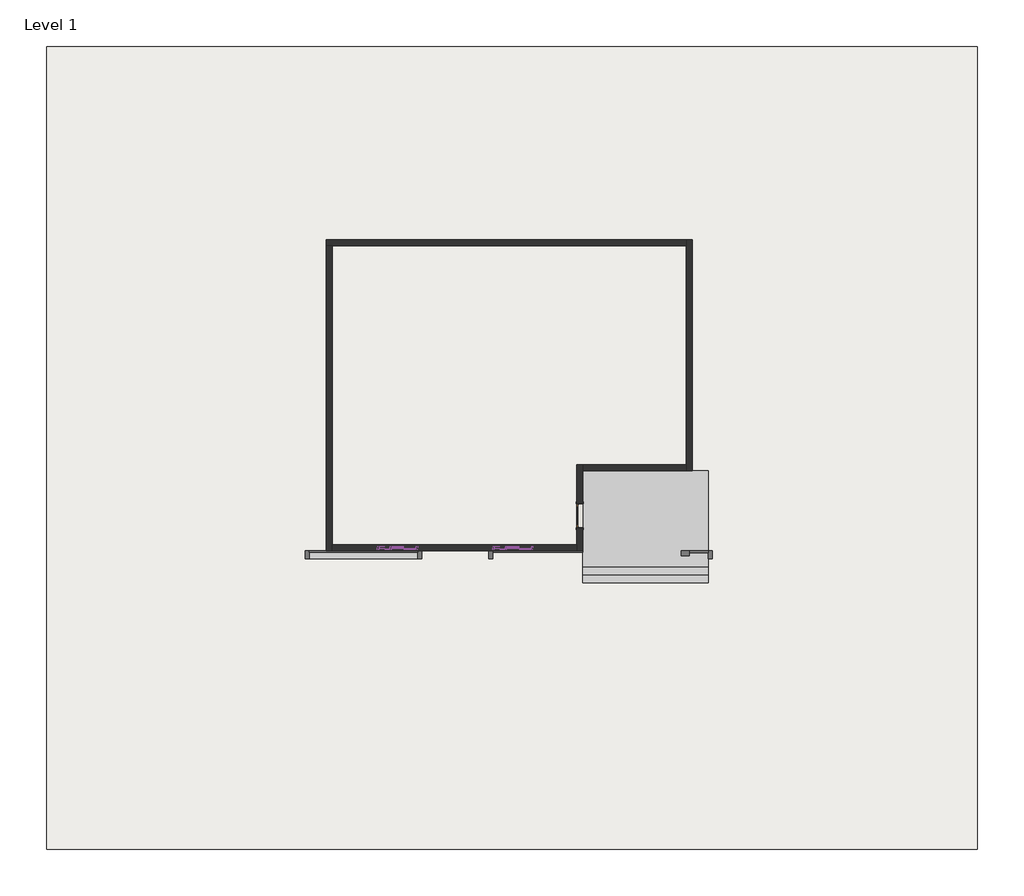
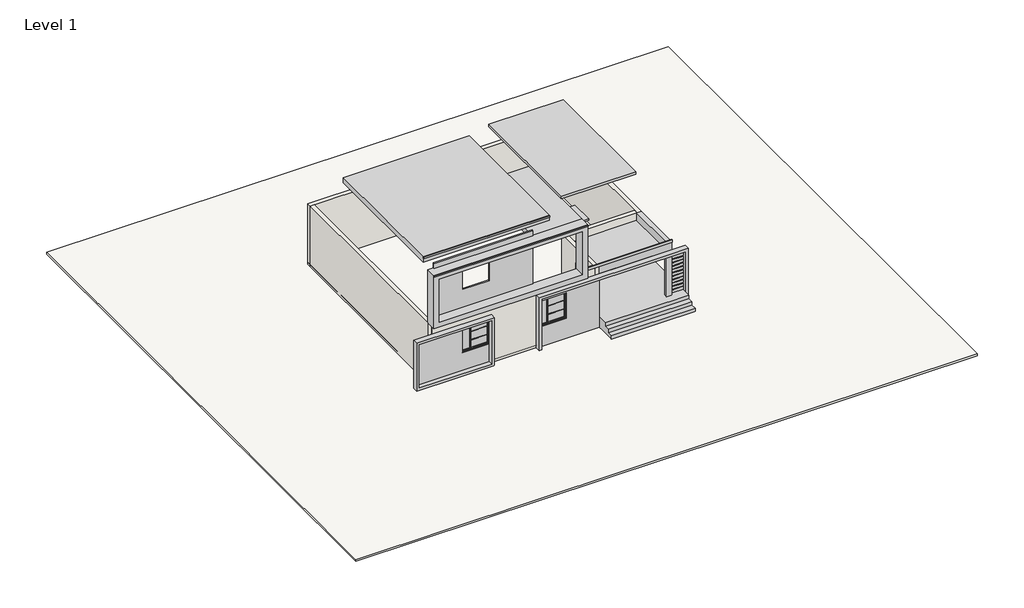
# One storey: 30 members, 8 plates, 6 walls, 2 slabs, 1 door, 1 proxy.
"""IFC4 building model written with IfcOpenShell, lengths in millimetres."""

from ifc_helpers import new_model, si_unit, frame, origin, origin_with_axes, place, context, project, spatial, polyline, outline, extrude, faceted_brep, transform, mapped, element, save
from components import generic_models_1_generic_models_1_b41e56dc, door_interior_single_1_panel_wood_4_x7_868ee8a9, member_c9b54d35, member_90750a43, member_dc106669, member_ff82125d, member_7fd687a9, system_panel_glazed_5efa86ec, system_panel_glazed_26b8bff8, system_panel_glazed_31531e99

model = new_model("IFC4")

# Units and contexts
model_context = context("Model", 3, world=origin())
ifc_project = project(units=[si_unit("LENGTHUNIT", "METRE", prefix="MILLI")], contexts=[model_context])

# Site, building, storey
site = spatial("IfcSite", under=ifc_project)
building = spatial("IfcBuilding", under=site)
storey = spatial("IfcBuildingStorey", under=building, Name="Level 1", Elevation=0.0)

# Proxy
placement = place(None, origin())
generic_models_1_generic_models_1_shape = generic_models_1_generic_models_1_b41e56dc(model_context)
element("IfcBuildingElementProxy", 1, Name="Generic Models 1 : Generic Models 1", ObjectType="Generic Models 1 : Generic Models 1", at=placement, inside=storey, context=model_context, shape_type="MappedRepresentation", body=[
    mapped(generic_models_1_generic_models_1_shape, transform((0.0, 0.0, 0.0), x_axis=(1.0, 0.0, 0.0), y_axis=(0.0, 1.0, 0.0), z_axis=(0.0, 0.0, 1.0))),
])

# Door
door_interior_single_1_panel_wood_4_x7_shape = door_interior_single_1_panel_wood_4_x7_868ee8a9(model_context)
element("IfcDoor", 2, ObjectType="Door-Interior-Single-1_Panel-Wood : 4'x7'", at=placement, inside=storey, context=model_context, shape_type="MappedRepresentation", body=[
    mapped(door_interior_single_1_panel_wood_4_x7_shape, transform((1261.9006121, -1809.8883122, 609.6), x_axis=(0.0, -1.0, 0.0), y_axis=(1.0, 0.0, 0.0), z_axis=(0.0, 0.0, 1.0))),
])

# Members
member_shape = member_c9b54d35(model_context)
element("IfcMember", 3, ObjectType="Rectangular Mullion : 1.5\" x 2.5\" rectangular", at=placement, inside=storey, context=model_context, shape_type="MappedRepresentation", body=[
    mapped(member_shape, transform((-5878.6743879, -3029.0883122, 2235.2), x_axis=(0.0, 0.0, 1.0), y_axis=(0.0, 1.0, 0.0), z_axis=(-1.0, 0.0, 0.0))),
])
element("IfcMember", 4, ObjectType="Rectangular Mullion : 1.5\" x 2.5\" rectangular", at=placement, inside=storey, context=model_context, shape_type="MappedRepresentation", body=[
    mapped(member_shape, transform((-5878.6743879, -3029.0883122, 1727.2), x_axis=(0.0, 0.0, 1.0), y_axis=(0.0, 1.0, 0.0), z_axis=(-1.0, 0.0, 0.0))),
])
element("IfcMember", 5, ObjectType="Rectangular Mullion : 1.5\" x 2.5\" rectangular", at=placement, inside=storey, context=model_context, shape_type="MappedRepresentation", body=[
    mapped(member_shape, transform((-1497.1743879, -3029.0883122, 2235.2), x_axis=(0.0, 0.0, 1.0), y_axis=(0.0, 1.0, 0.0), z_axis=(-1.0, 0.0, 0.0))),
])
element("IfcMember", 6, ObjectType="Rectangular Mullion : 1.5\" x 2.5\" rectangular", at=placement, inside=storey, context=model_context, shape_type="MappedRepresentation", body=[
    mapped(member_shape, transform((-1497.1743879, -3029.0883122, 1727.2), x_axis=(0.0, 0.0, 1.0), y_axis=(0.0, 1.0, 0.0), z_axis=(-1.0, 0.0, 0.0))),
])
member_2_shape = member_90750a43(model_context)
element("IfcMember", 7, ObjectType="Rectangular Mullion : 2.5\" x 5\" rectangular", at=placement, inside=storey, context=model_context, shape_type="MappedRepresentation", body=[
    mapped(member_2_shape, transform((-5910.4243879, -3029.0883122, 1727.2), x_axis=(-1.0, 0.0, 0.0), y_axis=(0.0, 1.0, 0.0), z_axis=(0.0, 0.0, -1.0))),
])
element("IfcMember", 8, ObjectType="Rectangular Mullion : 2.5\" x 5\" rectangular", at=placement, inside=storey, context=model_context, shape_type="MappedRepresentation", body=[
    mapped(member_2_shape, transform((-1528.9243879, -3029.0883122, 1727.2), x_axis=(-1.0, 0.0, 0.0), y_axis=(0.0, 1.0, 0.0), z_axis=(0.0, 0.0, -1.0))),
])
element("IfcMember", 9, ObjectType="Rectangular Mullion : 2.5\" x 5\" rectangular", at=placement, inside=storey, context=model_context, shape_type="MappedRepresentation", body=[
    mapped(member_2_shape, transform((-5910.4243879, -3029.0883122, 2235.2), x_axis=(-1.0, 0.0, 0.0), y_axis=(0.0, 1.0, 0.0), z_axis=(0.0, 0.0, -1.0))),
])
element("IfcMember", 10, ObjectType="Rectangular Mullion : 2.5\" x 5\" rectangular", at=placement, inside=storey, context=model_context, shape_type="MappedRepresentation", body=[
    mapped(member_2_shape, transform((-1528.9243879, -3029.0883122, 2235.2), x_axis=(-1.0, 0.0, 0.0), y_axis=(0.0, 1.0, 0.0), z_axis=(0.0, 0.0, -1.0))),
])
element("IfcMember", 11, ObjectType="Rectangular Mullion : 2.5\" x 5\" rectangular", at=placement, inside=storey, context=model_context, shape_type="MappedRepresentation", body=[
    mapped(member_2_shape, transform((-5910.4243879, -3029.0883122, 1219.2), x_axis=(-1.0, 0.0, 0.0), y_axis=(0.0, 1.0, 0.0), z_axis=(0.0, 0.0, -1.0))),
])
element("IfcMember", 12, ObjectType="Rectangular Mullion : 2.5\" x 5\" rectangular", at=placement, inside=storey, context=model_context, shape_type="MappedRepresentation", body=[
    mapped(member_2_shape, transform((-1528.9243879, -3029.0883122, 1219.2), x_axis=(-1.0, 0.0, 0.0), y_axis=(0.0, 1.0, 0.0), z_axis=(0.0, 0.0, -1.0))),
])
member_3_shape = member_dc106669(model_context)
element("IfcMember", 13, ObjectType="Rectangular Mullion : 2.5\" x 5\" rectangular", at=placement, inside=storey, context=model_context, shape_type="MappedRepresentation", body=[
    mapped(member_3_shape, transform((-6354.9243879, -3029.0883122, 2743.2), x_axis=(0.0, 0.0, 1.0), y_axis=(0.0, 1.0, 0.0), z_axis=(-1.0, 0.0, 0.0))),
])
element("IfcMember", 14, ObjectType="Rectangular Mullion : 2.5\" x 5\" rectangular", at=placement, inside=storey, context=model_context, shape_type="MappedRepresentation", body=[
    mapped(member_3_shape, transform((-1973.4243879, -3029.0883122, 2743.2), x_axis=(0.0, 0.0, 1.0), y_axis=(0.0, 1.0, 0.0), z_axis=(-1.0, 0.0, 0.0))),
])
member_4_shape = member_ff82125d(model_context)
element("IfcMember", 15, ObjectType="Rectangular Mullion : 2.5\" x 5\" rectangular", at=placement, inside=storey, context=model_context, shape_type="MappedRepresentation", body=[
    mapped(member_4_shape, transform((-4957.9243879, -3029.0883122, 1219.2), x_axis=(0.0, 0.0, -1.0), y_axis=(0.0, 1.0, 0.0), z_axis=(1.0, 0.0, 0.0))),
])
element("IfcMember", 16, ObjectType="Rectangular Mullion : 2.5\" x 5\" rectangular", at=placement, inside=storey, context=model_context, shape_type="MappedRepresentation", body=[
    mapped(member_4_shape, transform((-576.4243879, -3029.0883122, 1219.2), x_axis=(0.0, 0.0, -1.0), y_axis=(0.0, 1.0, 0.0), z_axis=(1.0, 0.0, 0.0))),
])
element("IfcMember", 17, ObjectType="Rectangular Mullion : 2.5\" x 5\" rectangular", at=placement, inside=storey, context=model_context, shape_type="MappedRepresentation", body=[
    mapped(member_3_shape, transform((-5942.1743879, -3029.0883122, 1219.2), x_axis=(0.0, 0.0, -1.0), y_axis=(0.0, 1.0, 0.0), z_axis=(1.0, 0.0, 0.0))),
])
element("IfcMember", 18, ObjectType="Rectangular Mullion : 2.5\" x 5\" rectangular", at=placement, inside=storey, context=model_context, shape_type="MappedRepresentation", body=[
    mapped(member_3_shape, transform((-1560.6743879, -3029.0883122, 1219.2), x_axis=(0.0, 0.0, -1.0), y_axis=(0.0, 1.0, 0.0), z_axis=(1.0, 0.0, 0.0))),
])
element("IfcMember", 19, ObjectType="Rectangular Mullion : 2.5\" x 5\" rectangular", at=placement, inside=storey, context=model_context, shape_type="MappedRepresentation", body=[
    mapped(member_4_shape, transform((-5878.6743879, -3029.0883122, 2743.2), x_axis=(0.0, 0.0, 1.0), y_axis=(0.0, 1.0, 0.0), z_axis=(-1.0, 0.0, 0.0))),
])
element("IfcMember", 20, ObjectType="Rectangular Mullion : 2.5\" x 5\" rectangular", at=placement, inside=storey, context=model_context, shape_type="MappedRepresentation", body=[
    mapped(member_4_shape, transform((-1497.1743879, -3029.0883122, 2743.2), x_axis=(0.0, 0.0, 1.0), y_axis=(0.0, 1.0, 0.0), z_axis=(-1.0, 0.0, 0.0))),
])
member_5_shape = member_7fd687a9(model_context)
element("IfcMember", 21, ObjectType="Rectangular Mullion : 2.5\" x 5\" rectangular", at=placement, inside=storey, context=model_context, shape_type="MappedRepresentation", body=[
    mapped(member_5_shape, transform((-4894.4243879, -3029.0883122, 2743.2), x_axis=(1.0, 0.0, 0.0), y_axis=(0.0, 1.0, 0.0), z_axis=(0.0, 0.0, 1.0))),
])
element("IfcMember", 22, ObjectType="Rectangular Mullion : 2.5\" x 5\" rectangular", at=placement, inside=storey, context=model_context, shape_type="MappedRepresentation", body=[
    mapped(member_5_shape, transform((-512.9243879, -3029.0883122, 2743.2), x_axis=(1.0, 0.0, 0.0), y_axis=(0.0, 1.0, 0.0), z_axis=(0.0, 0.0, 1.0))),
])
element("IfcMember", 23, ObjectType="Rectangular Mullion : 2.5\" x 5\" rectangular", at=placement, inside=storey, context=model_context, shape_type="MappedRepresentation", body=[
    mapped(member_5_shape, transform((-6418.4243879, -3029.0883122, 1219.2), x_axis=(-1.0, 0.0, 0.0), y_axis=(0.0, 1.0, 0.0), z_axis=(0.0, 0.0, -1.0))),
])
element("IfcMember", 24, ObjectType="Rectangular Mullion : 2.5\" x 5\" rectangular", at=placement, inside=storey, context=model_context, shape_type="MappedRepresentation", body=[
    mapped(member_5_shape, transform((-2036.9243879, -3029.0883122, 1219.2), x_axis=(-1.0, 0.0, 0.0), y_axis=(0.0, 1.0, 0.0), z_axis=(0.0, 0.0, -1.0))),
])
element("IfcMember", 25, ObjectType="Rectangular Mullion : 2.5\" x 5\" rectangular", at=placement, inside=storey, context=model_context, shape_type="MappedRepresentation", body=[
    mapped(member_5_shape, transform((-6418.4243879, -3029.0883122, 2235.2), x_axis=(-1.0, 0.0, 0.0), y_axis=(0.0, 1.0, 0.0), z_axis=(0.0, 0.0, -1.0))),
])
element("IfcMember", 26, ObjectType="Rectangular Mullion : 2.5\" x 5\" rectangular", at=placement, inside=storey, context=model_context, shape_type="MappedRepresentation", body=[
    mapped(member_5_shape, transform((-2036.9243879, -3029.0883122, 2235.2), x_axis=(-1.0, 0.0, 0.0), y_axis=(0.0, 1.0, 0.0), z_axis=(0.0, 0.0, -1.0))),
])
element("IfcMember", 27, ObjectType="Rectangular Mullion : 2.5\" x 5\" rectangular", at=placement, inside=storey, context=model_context, shape_type="MappedRepresentation", body=[
    mapped(member_5_shape, transform((-6418.4243879, -3029.0883122, 1727.2), x_axis=(-1.0, 0.0, 0.0), y_axis=(0.0, 1.0, 0.0), z_axis=(0.0, 0.0, -1.0))),
])
element("IfcMember", 28, ObjectType="Rectangular Mullion : 2.5\" x 5\" rectangular", at=placement, inside=storey, context=model_context, shape_type="MappedRepresentation", body=[
    mapped(member_5_shape, transform((-2036.9243879, -3029.0883122, 1727.2), x_axis=(-1.0, 0.0, 0.0), y_axis=(0.0, 1.0, 0.0), z_axis=(0.0, 0.0, -1.0))),
])
element("IfcMember", 29, ObjectType="Rectangular Mullion : 2.5\" x 5\" rectangular", at=placement, inside=storey, context=model_context, shape_type="MappedRepresentation", body=[
    mapped(member_5_shape, transform((-4894.4243879, -3029.0883122, 2235.2), x_axis=(1.0, 0.0, 0.0), y_axis=(0.0, 1.0, 0.0), z_axis=(0.0, 0.0, 1.0))),
])
element("IfcMember", 30, ObjectType="Rectangular Mullion : 2.5\" x 5\" rectangular", at=placement, inside=storey, context=model_context, shape_type="MappedRepresentation", body=[
    mapped(member_5_shape, transform((-512.9243879, -3029.0883122, 2235.2), x_axis=(1.0, 0.0, 0.0), y_axis=(0.0, 1.0, 0.0), z_axis=(0.0, 0.0, 1.0))),
])
element("IfcMember", 31, ObjectType="Rectangular Mullion : 2.5\" x 5\" rectangular", at=placement, inside=storey, context=model_context, shape_type="MappedRepresentation", body=[
    mapped(member_5_shape, transform((-4894.4243879, -3029.0883122, 1727.2), x_axis=(1.0, 0.0, 0.0), y_axis=(0.0, 1.0, 0.0), z_axis=(0.0, 0.0, 1.0))),
])
element("IfcMember", 32, ObjectType="Rectangular Mullion : 2.5\" x 5\" rectangular", at=placement, inside=storey, context=model_context, shape_type="MappedRepresentation", body=[
    mapped(member_5_shape, transform((-512.9243879, -3029.0883122, 1727.2), x_axis=(1.0, 0.0, 0.0), y_axis=(0.0, 1.0, 0.0), z_axis=(0.0, 0.0, 1.0))),
])

# Plates
system_panel_glazed_shape = system_panel_glazed_5efa86ec(model_context)
element("IfcPlate", 33, ObjectType="System Panel : Glazed", at=placement, inside=storey, context=model_context, shape_type="MappedRepresentation", body=[
    mapped(system_panel_glazed_shape, transform((-1036.7993879, -3029.0883122, 1282.7), x_axis=(-1.0, 0.0, 0.0), y_axis=(0.0, -1.0, 0.0), z_axis=(0.0, 0.0, 1.0))),
])
element("IfcPlate", 34, ObjectType="System Panel : Glazed", at=placement, inside=storey, context=model_context, shape_type="MappedRepresentation", body=[
    mapped(system_panel_glazed_shape, transform((-5418.2993879, -3029.0883122, 1282.7), x_axis=(-1.0, 0.0, 0.0), y_axis=(0.0, -1.0, 0.0), z_axis=(0.0, 0.0, 1.0))),
])
element("IfcPlate", 35, ObjectType="System Panel : Glazed", at=placement, inside=storey, context=model_context, shape_type="MappedRepresentation", body=[
    mapped(system_panel_glazed_shape, transform((-5418.2993879, -3029.0883122, 2254.25), x_axis=(-1.0, 0.0, 0.0), y_axis=(0.0, -1.0, 0.0), z_axis=(0.0, 0.0, 1.0))),
])
element("IfcPlate", 36, ObjectType="System Panel : Glazed", at=placement, inside=storey, context=model_context, shape_type="MappedRepresentation", body=[
    mapped(system_panel_glazed_shape, transform((-1036.7993879, -3029.0883122, 2254.25), x_axis=(-1.0, 0.0, 0.0), y_axis=(0.0, -1.0, 0.0), z_axis=(0.0, 0.0, 1.0))),
])
system_panel_glazed_2_shape = system_panel_glazed_26b8bff8(model_context)
element("IfcPlate", 37, ObjectType="System Panel : Glazed", at=placement, inside=storey, context=model_context, shape_type="MappedRepresentation", body=[
    mapped(system_panel_glazed_2_shape, transform((-6148.5493879, -3029.0883122, 1282.7), x_axis=(-1.0, 0.0, 0.0), y_axis=(0.0, -1.0, 0.0), z_axis=(0.0, 0.0, 1.0))),
])
element("IfcPlate", 38, ObjectType="System Panel : Glazed", at=placement, inside=storey, context=model_context, shape_type="MappedRepresentation", body=[
    mapped(system_panel_glazed_2_shape, transform((-1767.0493879, -3029.0883122, 1282.7), x_axis=(-1.0, 0.0, 0.0), y_axis=(0.0, -1.0, 0.0), z_axis=(0.0, 0.0, 1.0))),
])
system_panel_glazed_3_shape = system_panel_glazed_31531e99(model_context)
element("IfcPlate", 39, ObjectType="System Panel : Glazed", at=placement, inside=storey, context=model_context, shape_type="MappedRepresentation", body=[
    mapped(system_panel_glazed_3_shape, transform((-5418.2993879, -3029.0883122, 1746.25), x_axis=(-1.0, 0.0, 0.0), y_axis=(0.0, -1.0, 0.0), z_axis=(0.0, 0.0, 1.0))),
])
element("IfcPlate", 40, ObjectType="System Panel : Glazed", at=placement, inside=storey, context=model_context, shape_type="MappedRepresentation", body=[
    mapped(system_panel_glazed_3_shape, transform((-1036.7993879, -3029.0883122, 1746.25), x_axis=(-1.0, 0.0, 0.0), y_axis=(0.0, -1.0, 0.0), z_axis=(0.0, 0.0, 1.0))),
])

# Slabs
element("IfcSlab", 41, ObjectType="4\" floor", at=placement, inside=storey, context=model_context, shape_type="SweptSolid", body=[
    extrude(outline(polyline([(16371.8639765, 16010.8782458), (16371.8639765, -14469.1217542), (-18984.9360235, -14469.1217542), (-18984.9360235, 16010.8782458), (16371.8639765, 16010.8782458)])), frame((0.0, 0.0, -101.6), z_axis=(0.0, 0.0, 1.0), x_axis=(1.0, 0.0, 0.0)), (0.0, 0.0, 1.0), 101.6),
])
element("IfcSlab", 42, ObjectType="6\" GF", at=placement, inside=storey, context=model_context, shape_type="SweptSolid", body=[
    extrude(outline(polyline([(5532.2756121, 8667.6116878), (5532.2756121, -3143.3883122), (-8361.5243879, -3143.3883122), (-8361.5243879, 8667.6116878), (5532.2756121, 8667.6116878)])), origin_with_axes(), (0.0, 0.0, 1.0), 152.4),
])

# Walls
element("IfcWall", 43, ObjectType="9\" wall", at=placement, inside=storey, context=model_context, shape_type="Brep", body=[
    faceted_brep([(-8361.5243879, 8439.0116878, 0.0), (-8132.9243879, 8439.0116878, 0.0), (5303.6756121, 8439.0116878, 0.0), (5303.6756121, 8439.0116878, 3657.6), (-8132.9243879, 8439.0116878, 3657.6), (-8361.5243879, 8439.0116878, 3657.6), (-8361.5243879, 8667.6116878, 0.0), (-8361.5243879, 8667.6116878, 3657.6), (5303.6756121, 8667.6116878, 3657.6), (5303.6756121, 8667.6116878, 0.0)], [[[0, 1, 2, 3, 4, 5]], [[6, 7, 8, 9]], [[2, 1, 0, 6, 9]], [[5, 4, 3, 8, 7]], [[0, 5, 7, 6]], [[3, 2, 9, 8]]]),
])
element("IfcWall", 44, ObjectType="9\" wall", at=placement, inside=storey, context=model_context, shape_type="Brep", body=[
    faceted_brep([(-8132.9243879, -3143.3883122, 0.0), (-8132.9243879, -2914.7883122, 0.0), (-8132.9243879, 8439.0116878, 0.0), (-8132.9243879, 8439.0116878, 3657.6), (-8132.9243879, -2914.7883122, 3657.6), (-8132.9243879, -3143.3883122, 3657.6), (-8361.5243879, -3143.3883122, 0.0), (-8361.5243879, -3143.3883122, 3657.6), (-8361.5243879, 8439.0116878, 3657.6), (-8361.5243879, 8439.0116878, 0.0)], [[[0, 1, 2, 3, 4, 5]], [[6, 7, 8, 9]], [[2, 1, 0, 6, 9]], [[5, 4, 3, 8, 7]], [[0, 5, 7, 6]], [[3, 2, 9, 8]]]),
])
element("IfcWall", 45, ObjectType="9\" wall", at=placement, inside=storey, context=model_context, shape_type="Brep", body=[
    faceted_brep([(5303.6756121, 8667.6116878, 0.0), (5303.6756121, 8439.0116878, 0.0), (5303.6756121, 133.2116878, 0.0), (5303.6756121, -95.3883122, 0.0), (5303.6756121, -95.3883122, 3657.6), (5303.6756121, 133.2116878, 3657.6), (5303.6756121, 8439.0116878, 3657.6), (5303.6756121, 8667.6116878, 3657.6), (5532.2756121, 8667.6116878, 0.0), (5532.2756121, 8667.6116878, 3657.6), (5532.2756121, -95.3883122, 3657.6), (5532.2756121, -95.3883122, 0.0)], [[[0, 1, 2, 3, 4, 5, 6, 7]], [[8, 9, 10, 11]], [[3, 2, 1, 0, 8, 11]], [[7, 6, 5, 4, 10, 9]], [[0, 7, 9, 8]], [[4, 3, 11, 10]]]),
])
element("IfcWall", 46, ObjectType="9\" wall", at=placement, inside=storey, context=model_context, shape_type="Brep", body=[
    faceted_brep([(1379.3756121, -3143.3883122, 0.0), (1379.3756121, -95.3883122, 0.0), (1379.3756121, 133.2116878, 0.0), (1379.3756121, 133.2116878, 3657.6), (1379.3756121, -95.3883122, 3657.6), (1379.3756121, -3143.3883122, 3657.6), (1379.3756121, -2292.4883122, 609.6), (1379.3756121, -2292.4883122, 2768.6), (1379.3756121, -1327.2883122, 2768.6), (1379.3756121, -1327.2883122, 609.6), (1150.7756121, 133.2116878, 0.0), (1150.7756121, -2914.7883122, 0.0), (1150.7756121, -3143.3883122, 0.0), (1150.7756121, -3143.3883122, 3657.6), (1150.7756121, -2914.7883122, 3657.6), (1150.7756121, 133.2116878, 3657.6), (1150.7756121, -2292.4883122, 2768.6), (1150.7756121, -2292.4883122, 609.6), (1150.7756121, -1327.2883122, 609.6), (1150.7756121, -1327.2883122, 2768.6)], [[[0, 1, 2, 3, 4, 5], [6, 7, 8, 9]], [[10, 11, 12, 13, 14, 15], [16, 17, 18, 19]], [[2, 1, 0, 12, 11, 10]], [[5, 4, 3, 15, 14, 13]], [[3, 2, 10, 15]], [[0, 5, 13, 12]], [[6, 17, 16, 7]], [[7, 16, 19, 8]], [[8, 19, 18, 9]], [[17, 6, 9, 18]]]),
])
element("IfcWall", 47, ObjectType="9\" wall", at=placement, inside=storey, context=model_context, shape_type="SweptSolid", body=[
    extrude(outline(polyline([(5303.6756121, -95.3883122), (1379.3756121, -95.3883122), (1379.3756121, 133.2116878), (5303.6756121, 133.2116878), (5303.6756121, -95.3883122)])), origin_with_axes(), (0.0, 0.0, 1.0), 3657.6),
])
element("IfcWall", 48, ObjectType="9\" wall", at=placement, inside=storey, context=model_context, shape_type="SweptSolid", body=[
    extrude(outline(polyline([(0.0, -8132.9243879), (0.0, 1150.7756121), (3657.6, 1150.7756121), (3657.6, -8132.9243879), (0.0, -8132.9243879)]), holes=[polyline([(2743.2, -4894.4243879), (1219.2, -4894.4243879), (1219.2, -6418.4243879), (2743.2, -6418.4243879), (2743.2, -4894.4243879)]), polyline([(2743.2, -512.9243879), (1219.2, -512.9243879), (1219.2, -2036.9243879), (2743.2, -2036.9243879), (2743.2, -512.9243879)])]), frame((0.0, -3143.3883122, 0.0), z_axis=(0.0, 1.0, 0.0), x_axis=(0.0, 0.0, 1.0)), (0.0, 0.0, 1.0), 228.6),
])

save(model, "model.ifc")

# Revit data of these elements
# Type "Door-Interior-Single-1_Panel-Wood : 4'x7'"
#   Type Mark = "9"
#   Assembly Code = "C1020300"
#   Analytic Construction = "Wooden"
#   Top Rail = 0' - 4 11/16"
#   Thickness = 0' - 1 3/8"
#   Thermal Resistance (R) = 2.5876 (h·ft²·°F)/BTU
#   Swing Angle [instance default] = 90.00°
#   Stiles = 0' - 4 3/4"
#   Rough Width = 3' - 2"
#   Rough Height = 7' - 1"
#   Height = 7' - 0"
#   Width = 3' - 0"
#   Heat Transfer Coefficient (U) = 0.3865 BTU/(h·ft²·°F)
#   Bottom Rail = 0' - 9 1/8"
#   Trim Material = Cherry
#   Panel Material = Cherry
#   Frame Material = Cherry
#   Door Handle Material = Aluminum
#   Visual Light Transmittance = 0
#   Solar Heat Gain Coefficient = 0
#   Wall Closure = (empty or 0)
#   Function = (empty or 0)
# Type "Rectangular Mullion : 1.5\" x 2.5\" rectangular"
#   built-in parameter 1007304 = 0.208333 (stored number, unit not read)
#   built-in parameter 1007301 = 0.0625 (stored number, unit not read)
#   built-in parameter 1007300 = 0.0625 (stored number, unit not read)
# Type "Rectangular Mullion : 2.5\" x 5\" rectangular"
#   built-in parameter 1007304 = 0.416667 (stored number, unit not read)
#   built-in parameter 1007301 = 0.104167 (stored number, unit not read)
#   built-in parameter 1007300 = 0.104167 (stored number, unit not read)
# Type "System Panel : Glazed"
#   Construction Type Id = "GSP4R"
#   Analytic Construction = "1/8 in Pilkington single glazing"
#   Visual Light Transmittance = 0.9
#   Solar Heat Gain Coefficient = 0.86
#   Heat Transfer Coefficient (U) = 1.18115 BTU/(h·ft²·°F)
#   Define Thermal Properties by = 1
# Type "4\" floor"
#   Assembly Code = "B1010"
#   Function = 0
# Type "6\" GF"
#   Assembly Code = "B1010"
#   Function = 0
#   Layers, outside or top first: 0' - 6" no material (function 1)
# Type "9\" wall"
#   Assembly Code = "B2010"
#   Layers, outside or top first: 0' - 9" no material (function 1)
# Element 1 (IfcBuildingElementProxy, "Generic Models 1 : Generic Models 1")
#   Phase Created = New Construction
#   Materials on its faces: "Gypsum Wall Board", "Clad - White", "Wood Planks", "Ash colour"
# Element 2 (IfcDoor, "Door-Interior-Single-1_Panel-Wood : 4'x7'")
#   Swing Angle = 90.00°
#   Phase Created = New Construction
#   Materials on its faces: "Cherry", "Aluminum"
# Elements 3, 4, 5, 6 (IfcMember, "Rectangular Mullion : 1.5\" x 2.5\" rectangular")
#   Phase Created = New Construction
# Elements 7, 8, 9, 10, 11, 12, 13, 14, 15, 16, 17, 18, 19, 20, 21, 22, 23, 24, 25, 26, 27, 28, 29, 30, 31, 32 (IfcMember, "Rectangular Mullion : 2.5\" x 5\" rectangular")
#   Phase Created = New Construction
# Elements 33, 34, 35, 36, 37, 38, 39, 40 (IfcPlate, "System Panel : Glazed")
#   Phase Created = New Construction
#   Materials on its faces: "Glass"
# Element 41 (IfcSlab, "4\" floor")
#   Height Offset From Level = 0' - 0"
#   Phase Created = New Construction
# Element 42 (IfcSlab, "6\" GF")
#   Height Offset From Level = 0' - 6"
#   Phase Created = New Construction
#   Materials on its faces: "Default Floor"
# Elements 43, 44, 45, 46, 47, 48 (IfcWall, "9\" wall")
#   Top Offset = 0' - 0"
#   Base Offset = 0' - 0"
#   wall height = 12' - 0"
#   Phase Created = New Construction
#   Base Constraint = Level 1
#   Top Constraint = Level 2
#   Materials on its faces: "Default Wall"
# Materials
#   "Cherry": class "Wood", colour RGB 226 177 128, transparency 0, Description = "Prunus Serotina", Cost = 0
#   "Aluminum": class "Metal", colour RGB 247 247 247, transparency 0, Description = "Aluminum 6061", Cost = 0
#   "Gypsum Wall Board": class "Generic", colour RGB 127 127 127, transparency 0, Description = "Gypsum Wall Board", Cost = 0
#   "Clad - White": class "Wood", colour RGB 242 242 238, transparency 0, Cost = 0
#   "Wood Planks": class "Wood", colour RGB 193 160 115, transparency 0, Description = "Physical material.", Cost = 0
#   "Ash colour": class "Generic", colour RGB 120 120 120, transparency 0, Cost = 0
#   "Glass": class "Glass", colour RGB 0 128 192, transparency 0.75, Description = "Soda Lime Glass", Cost = 0
#   "Default Floor": colour RGB 128 128 128, transparency 0, Cost = 0
#   "Default Wall": colour RGB 128 128 128, transparency 0, Cost = 0
